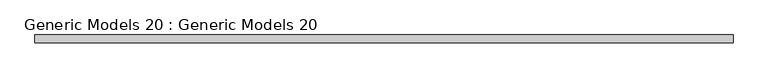
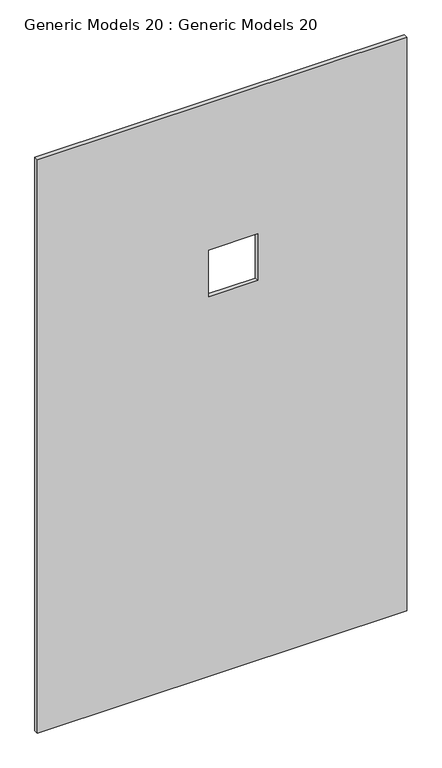
"""IFC4 building model written with IfcOpenShell, lengths in millimetres: proxy geometry, Generic Models 20 : Generic Models 20."""

from ifc_helpers import new_model, si_unit, frame, origin, place, context, project, spatial, polyline, outline, extrude, source, transform, mapped, element, save


def generic_models_20_generic_models_20_543834f7(model_context):
    return source(origin(), model_context, "Body", "SweptSolid", [
        extrude(outline(polyline([(7810.4767967, -2677.3781265), (304.8, -2677.3781265), (304.8, 1894.6218735), (7810.4767967, 1894.6218735), (7810.4767967, -2677.3781265)]), holes=[polyline([(5882.0336242, -556.4781265), (5882.0336242, 53.1218735), (5272.4336242, 53.1218735), (5272.4336242, -556.4781265), (5882.0336242, -556.4781265)])]), frame((0.0, 8336.1857468, 0.0), z_axis=(0.0, 1.0, 0.0), x_axis=(0.0, 0.0, 1.0)), (0.0, 0.0, 1.0), 50.8),
    ])


if __name__ == "__main__":
    model = new_model("IFC4")
    model_context = context("Model", 3, world=origin())
    ifc_project = project(units=[si_unit("LENGTHUNIT", "METRE", prefix="MILLI")], contexts=[model_context])
    site = spatial("IfcSite", under=ifc_project)
    building = spatial("IfcBuilding", under=site)
    placement = place(None, origin())
    generic_models_20_generic_models_20_shape = generic_models_20_generic_models_20_543834f7(model_context)
    element("IfcBuildingElementProxy", 1, Name="Generic Models 20 : Generic Models 20", ObjectType="Generic Models 20 : Generic Models 20", at=placement, inside=building, context=model_context, shape_type="MappedRepresentation", body=[
        mapped(generic_models_20_generic_models_20_shape, transform((0.0, 0.0, 0.0), x_axis=(1.0, 0.0, 0.0), y_axis=(0.0, 1.0, 0.0), z_axis=(0.0, 0.0, 1.0))),
    ])
    save(model, "model.ifc")

# Revit data of these elements
# Element 1 (IfcBuildingElementProxy, "Generic Models 20 : Generic Models 20")
#   Materials on its faces: "GOLD COLOUR"
# Materials
#   "GOLD COLOUR": class "Generic", colour RGB 120 120 120, transparency 0, Cost = 0
